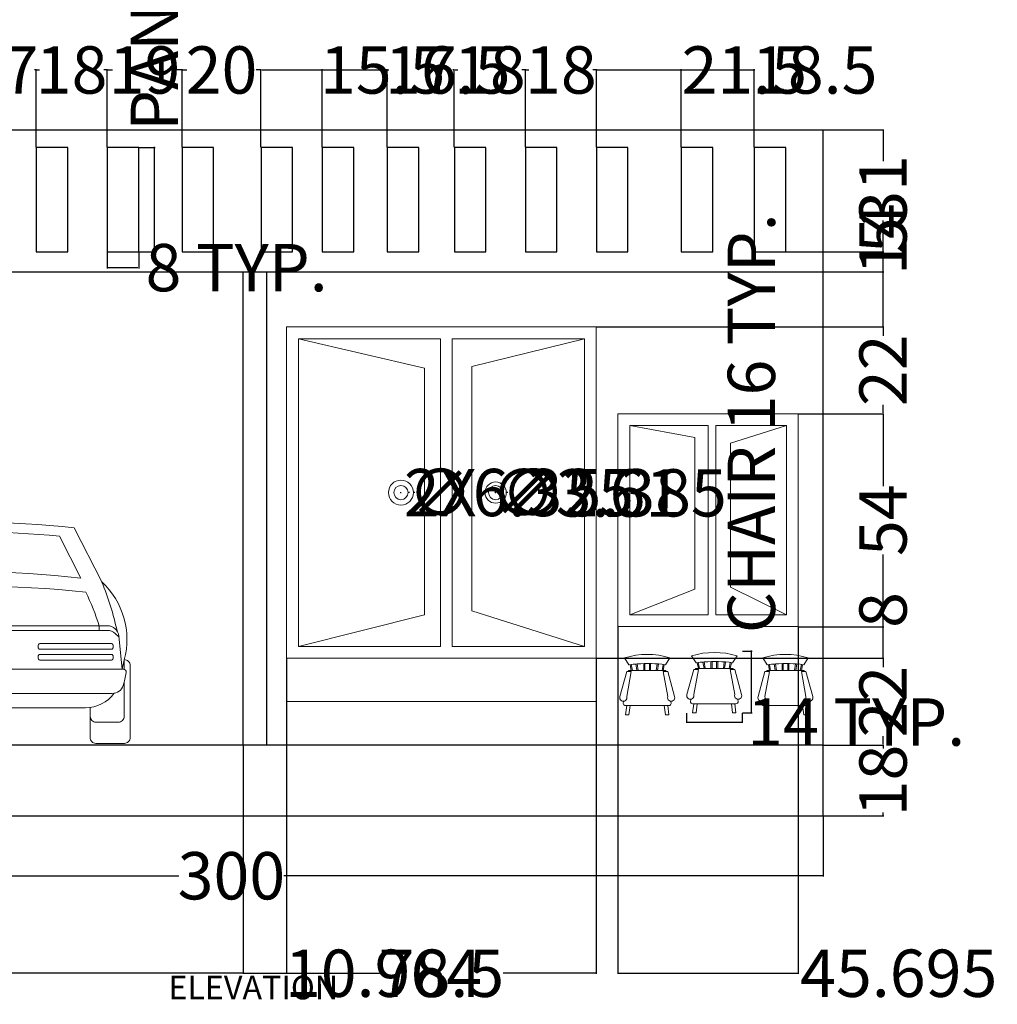
# Model space of a CAD drawing. Units: inches. Extents: x -101 to 786, y 26 to 880.
# Tile 7 of 9: x 538 to 786, y 45 to 295. Entities that reach past the tile are written whole.
import ezdxf

# ---------------------------------------------------------------- set-up
doc = ezdxf.new("R2010")
doc.units = ezdxf.units.IN
doc.header["$MEASUREMENT"] = 0
for name, color, linetype, lineweight in [('A-ANNO-DIMS', 2, 'Continuous', 18), ('A-ANNO-TEXT', 7, 'Continuous', 25), ('A-DOOR', 4, 'Continuous', 20), ('A-ELEV', 7, 'Continuous', 30), ('A-EQPM-VEHC', 9, 'Continuous', 13), ('A-FLOR-STRS', 7, 'Continuous', 20), ('A-FURN', 8, 'Continuous', 13), ('A-GLAZ', 4, 'Continuous', 18)]:
    doc.layers.add(name, color=color, linetype=linetype, lineweight=lineweight)
doc.styles.get("Standard").update_dxf_attribs({"font": 'arial.ttf'})
doc.dimstyles.get("Standard").update_dxf_attribs({"dimtxt": 12, "dimasz": 0.18, "dimexe": 0.18, "dimexo": 0.0625, "dimgap": 0.09, "dimtad": 0, "dimdec": 1, "dimzin": 0, "dimdsep": 46, "dimlunit": 3, "dimtxsty": 'Standard', "dimcen": 0.09, "dimadec": 0, "dimazin": 0, "dimtfac": 1, "dimtdec": 1, "dimtofl": 0, "dimtmove": 0, "dimatfit": 3, "dimfxl": 1, "dimtolj": 1, "dimtzin": 0, "dimarcsym": 0})

# ---------------------------------------------------------------- blocks, each defined once
blk = doc.blocks.new('*U16')
for p, q in [((-24.66, 54.68), (-31.66, 40.93)), ((31.66, 40.93), (24.66, 54.68)), ((-30.95, 37.96), (-30.95, 37.96)), ((-37.32, 21.22), (-36.82, 18.83)), ((36.82, 18.83), (37.31, 21.2)), ((-27.55, 9), (27.55, 9))]:
    blk.add_line(p, q)
for points in [[(-20.92, 52.5), (-26.31, 41.89), (-26.31, 41.89, -0.059427), (26.31, 41.89), (20.92, 52.5, 0.05217)], [(-34.12, 25.29), (-15.92, 25.29, -0.414214), (-15.55, 24.92), (-15.55, 24.24, -0.414214), (-15.92, 23.87), (-34.12, 23.87, -0.414214), (-34.49, 24.24), (-34.49, 24.92, -0.414214)], [(-2.82, 25.12), (2.9, 25.12, -0.414214), (3.64, 24.38), (3.64, 20.97, -0.414214), (2.9, 20.23), (-2.82, 20.23, -0.414214), (-3.56, 20.97), (-3.56, 24.38, -0.414214)], [(34.12, 25.29), (15.92, 25.29, 0.414214), (15.55, 24.92), (15.55, 24.24, 0.414214), (15.92, 23.87), (34.12, 23.87, 0.414214), (34.49, 24.24), (34.49, 24.92, 0.414214)], [(-34.12, 22.54), (-15.92, 22.54, -0.414214), (-15.55, 22.17), (-15.55, 21.49, -0.414214), (-15.92, 21.12), (-34.12, 21.12, -0.414214), (-34.49, 21.49), (-34.49, 22.17, -0.414214)], [(34.12, 22.54), (15.92, 22.54, 0.414214), (15.55, 22.17), (15.55, 21.49, 0.414214), (15.92, 21.12), (34.12, 21.12, 0.414214), (34.49, 21.49), (34.49, 22.17, 0.414214)], [(-7.5, 16.83, -0.414214), (-7, 17.33), (7, 17.33, -0.414214), (7.5, 16.83), (7.5, 13.67, 0.414214), (8.5, 12.67), (34.29, 12.67, 0.322734), (37.1, 14.69, 0.029256), (37.41, 15.83), (37.84, 17.94, 0.475639), (37.12, 18.83), (9, 18.83, -0.414214), (8.75, 19.08, 0.414214), (8.5, 19.33), (-8.5, 19.33, 0.414214), (-8.75, 19.08, -0.414214), (-9, 18.83), (-37.12, 18.83, 0.475639), (-37.84, 17.94), (-37.41, 15.83, 0.029158), (-37.1, 14.7, 0.322842), (-34.29, 12.67), (-8.5, 12.67, 0.414214), (-7.5, 13.67)]]:
    blk.add_lwpolyline(points, format="xyb", close=True)
for points in [[(30.95, 28.64), (30.95, 29.82, 0.037308), (27.62, 38.34, 0.052989), (-27.62, 38.34, 0.037308), (-30.95, 29.82), (-30.95, 28.64)], [(-36.82, 18.83), (-35.99, 27.2, -0.380946), (-33.05, 29.82), (33.04, 29.82, -0.380474), (35.98, 27.2), (36.82, 18.83)], [(-36.02, 26.89), (-35.02, 27.89, -0.184023), (-33.05, 28.64), (33.05, 28.64, -0.184023), (35.02, 27.89), (36.02, 26.89)], [(-28.73, 9.08), (-28.73, 1.48, -0.414214), (-30.21, 0), (-37.44, 0, -0.414214), (-38.92, 1.48), (-38.92, 19.74, -0.414214), (-37.44, 21.22), (-37.32, 21.22)], [(28.67, 9.07), (28.67, 1.48, 0.414214), (30.15, 0), (37.38, 0, 0.414214), (38.86, 1.48), (38.86, 19.74, 0.414214), (37.38, 21.22), (37.32, 21.22)], [(-37.32, 15.44), (-37.32, 6.85, 0.414214), (-35.84, 5.37), (-30.21, 5.37, 0.414214), (-28.73, 6.85), (-28.73, 9.08)], [(37.32, 15.44), (37.32, 6.85, -0.414214), (35.84, 5.37), (30.21, 5.37, -0.414214), (28.73, 6.85), (28.73, 9.08)]]:
    blk.add_lwpolyline(points, format="xyb")
for points in [[(-37.32, 21.22), (-37.32, 18.8)], [(37.32, 21.22), (37.32, 18.8)]]:
    blk.add_lwpolyline(points)
blk.add_circle((0, 26.18), 0.596)
for centre, radius, start, end in [((0, -181.13), 237.1, 84.03, 95.97), ((-18.4, 26.45), 19.63, 132.4835, 195.4658), ((30.86, 14.66), 67.81, 157.2124, 168.2366), ((18.26, 26.38), 19.77, 344.8595, 47.3598), ((-31.75, 14.41), 68.72, 11.827, 22.6625), ((-27.55, 17.88), 8.88, 215.5776, 270.0028), ((27.55, 17.88), 8.88, 270.0028, 324.3999)]:
    blk.add_arc(centre, radius, start, end)
blk = doc.blocks.new('Chair - Rocking')
for p, q in [((-8, -4.5), (-10, -1.5)), ((-4.5, -7), (-4.96674, -4.19951)), ((-4, -7), (-4.40532, -4.16272)), ((-1.5, -4.05012), (-1.5, -7)), ((-1, -7), (-1, -4.05012)), ((1, -7), (1, -4.04655)), ((1.5, -4.05012), (1.5, -7)), ((4, -7), (4.40187, -4.18694)), ((4.5, -7), (4.96761, -4.19437)), ((8, -4.5), (10, -1.5)), ((-9, -7.5), (-12, -18.49999)), ((-7, -7.5), (-9, -7.5)), ((-9, -18.49999), (-7, -7.5)), ((-8.23428, -6.99939), (-8.3093, -7.47958)), ((-8.23041, -7), (8.23915, -7)), ((-7.5, -4.5), (-7, -7)), ((-6.5, -7), (-7.02225, -4.43)), ((6.5, -7), (7, -4.4057)), ((7.5, -4.5), (7, -7)), ((7, -7.5), (9, -7.5)), ((9, -18.49999), (7, -7.5)), ((8.31071, -7.48854), (8.23449, -7.00073)), ((9, -7.5), (12, -18.49999)), ((-10.36644, -20.64523), (-10.5, -21.49999)), ((10.5, -21.49999), (10.3575, -20.58798)), ((-9, -22.49999), (-9.5, -26.49999)), ((0, -22.49999), (-9.5, -22.49999)), ((-8, -26.49999), (-7.5, -22.49999)), ((0, -22.49999), (9.5, -22.49999)), ((8, -26.49999), (7.5, -22.49999)), ((9, -22.49999), (9.5, -26.49999)), ((-9.5, -26.49999), (-8, -26.49999)), ((9.5, -26.49999), (8, -26.49999))]:
    blk.add_line(p, q)
for centre, radius, start, end in [((0, -34.08333), 34.08333, 72.93847, 107.0615), ((0, -68.25004), 64.25, 93.92211, 97.15267), ((0, -68.25004), 64.25, 82.84733, 93.92211), ((-10.5, -18.99999), 1.58114, 161.5651, 18.43495), ((-9.5, -21.49999), 1, 180, 270), ((10.5, -18.99999), 1.58114, 161.5651, 18.43495), ((9.5, -21.49999), 1, 270, 0)]:
    blk.add_arc(centre, radius, start, end)
blk = doc.blocks.new('PARAPET-PANEL-8')
blk.add_lwpolyline([(0, 0), (8, 0), (8, 26.5), (0, 26.5)], close=True)
blk = doc.blocks.new('*D27')
at = {"layer": 'A-ANNO-DIMS', "color": 0, "lineweight": -2, "transparency": 16777216}
for p, q in [((568.37, 262.42), (572.47, 262.42)), ((572.29, 262.42), (572.29, 262.6)), ((572.29, 236.1), (572.29, 262.24)), ((568.37, 235.92), (572.47, 235.92))]:
    blk.add_line(p, q, dxfattribs=at)
at = {"layer": 'A-ANNO-DIMS', "color": 0, "transparency": 16777216}
for points in [[(572.26, 262.24), (572.32, 262.24), (572.29, 262.42)], [(572.26, 236.1), (572.32, 236.1), (572.29, 235.92)]]:
    blk.add_solid(points, dxfattribs=at)
at = {"layer": 'Defpoints', "color": 0, "transparency": 16777216}
for p in [(568.31, 262.42), (572.29, 262.42), (568.31, 235.92)]:
    blk.add_point(p, dxfattribs=at)
at = {"layer": 'A-ANNO-DIMS', "color": 0, "transparency": 16777216, "insert": (572.29, 321.42), "char_height": 12, "attachment_point": 5, "rotation": 90}
blk.add_mtext('\\A1;PANEL 27 TYP.', dxfattribs=at)
blk = doc.blocks.new('*D28')
at = {"layer": 'A-ANNO-DIMS', "color": 0, "lineweight": -2, "transparency": 16777216}
for p, q in [((560.31, 235.86), (560.31, 231.77)), ((568.31, 235.86), (568.31, 231.77)), ((560.49, 231.95), (568.13, 231.95)), ((568.31, 231.95), (568.49, 231.95))]:
    blk.add_line(p, q, dxfattribs=at)
at = {"layer": 'A-ANNO-DIMS', "color": 0, "transparency": 16777216}
for points in [[(560.49, 231.98), (560.49, 231.92), (560.31, 231.95)], [(568.13, 231.98), (568.13, 231.92), (568.31, 231.95)]]:
    blk.add_solid(points, dxfattribs=at)
at = {"layer": 'Defpoints', "color": 0, "transparency": 16777216}
for p in [(560.31, 235.92), (568.31, 235.92), (568.31, 231.95)]:
    blk.add_point(p, dxfattribs=at)
at = {"layer": 'A-ANNO-DIMS', "color": 0, "transparency": 16777216, "insert": (593.13, 231.95), "char_height": 12, "attachment_point": 5}
blk.add_mtext('\\A1;8 TYP.', dxfattribs=at)
blk = doc.blocks.new('*D33')
at = {"layer": 'A-ANNO-DIMS', "color": 0, "lineweight": -2, "transparency": 16777216}
for p, q in [((723.59, 134.67), (723.59, 134.85)), ((721.31, 134.67), (723.77, 134.67)), ((723.59, 119.27), (723.59, 134.49)), ((721.31, 119.09), (723.77, 119.09))]:
    blk.add_line(p, q, dxfattribs=at)
at = {"layer": 'A-ANNO-DIMS', "color": 0, "transparency": 16777216}
for points in [[(723.56, 134.49), (723.62, 134.49), (723.59, 134.67)], [(723.56, 119.27), (723.62, 119.27), (723.59, 119.09)]]:
    blk.add_solid(points, dxfattribs=at)
at = {"layer": 'Defpoints', "color": 0, "transparency": 16777216}
for p in [(721.25, 134.67), (723.59, 134.67), (721.25, 119.09)]:
    blk.add_point(p, dxfattribs=at)
at = {"layer": 'A-ANNO-DIMS', "color": 0, "transparency": 16777216, "insert": (723.59, 192.49), "char_height": 12, "attachment_point": 5, "rotation": 90}
blk.add_mtext('\\A1;CHAIR 16 TYP.', dxfattribs=at)
blk = doc.blocks.new('*D34')
at = {"layer": 'A-ANNO-DIMS', "color": 0, "lineweight": -2, "transparency": 16777216}
for p, q in [((707.15, 119.02), (707.15, 116.57)), ((721.25, 119.02), (721.25, 116.57)), ((707.33, 116.75), (721.07, 116.75)), ((721.25, 116.75), (721.43, 116.75))]:
    blk.add_line(p, q, dxfattribs=at)
at = {"layer": 'A-ANNO-DIMS', "color": 0, "transparency": 16777216}
for points in [[(707.33, 116.78), (707.33, 116.72), (707.15, 116.75)], [(721.07, 116.78), (721.07, 116.72), (721.25, 116.75)]]:
    blk.add_solid(points, dxfattribs=at)
at = {"layer": 'Defpoints', "color": 0, "transparency": 16777216}
for p in [(707.15, 119.09), (721.25, 119.09), (721.25, 116.75)]:
    blk.add_point(p, dxfattribs=at)
at = {"layer": 'A-ANNO-DIMS', "color": 0, "transparency": 16777216, "insert": (750.16, 116.75), "char_height": 12, "attachment_point": 5}
blk.add_mtext('\\A1;14 TYP.', dxfattribs=at)
blk = doc.blocks.new('*D89')
at = {"layer": 'A-ANNO-DIMS', "color": 0, "lineweight": -2, "transparency": 16777216}
for p, q in [((441.81, 92.86), (441.81, 77.59)), ((741.81, 92.86), (741.81, 77.59)), ((441.99, 77.77), (578.49, 77.77)), ((741.63, 77.77), (605.13, 77.77))]:
    blk.add_line(p, q, dxfattribs=at)
at = {"layer": 'A-ANNO-DIMS', "color": 0, "transparency": 16777216}
for points in [[(441.99, 77.8), (441.99, 77.74), (441.81, 77.77)], [(741.63, 77.8), (741.63, 77.74), (741.81, 77.77)]]:
    blk.add_solid(points, dxfattribs=at)
at = {"layer": 'Defpoints', "color": 0, "transparency": 16777216}
for p in [(441.81, 92.92), (741.81, 92.92), (441.81, 77.77)]:
    blk.add_point(p, dxfattribs=at)
at = {"layer": 'A-ANNO-DIMS', "color": 0, "transparency": 16777216, "insert": (591.81, 77.77), "char_height": 12, "attachment_point": 5}
blk.add_mtext('\\A1;300', dxfattribs=at)
blk = doc.blocks.new('*D95')
at = {"layer": 'A-ANNO-DIMS', "color": 0, "lineweight": -2, "transparency": 16777216}
for p, q in [((525.31, 262.49), (525.31, 282.25)), ((542.31, 262.49), (542.31, 282.25)), ((525.49, 282.07), (525.69, 282.07)), ((542.13, 282.07), (541.93, 282.07))]:
    blk.add_line(p, q, dxfattribs=at)
at = {"layer": 'A-ANNO-DIMS', "color": 0, "transparency": 16777216}
for points in [[(525.49, 282.1), (525.49, 282.04), (525.31, 282.07)], [(542.13, 282.1), (542.13, 282.04), (542.31, 282.07)]]:
    blk.add_solid(points, dxfattribs=at)
at = {"layer": 'Defpoints', "color": 0, "transparency": 16777216}
for p in [(542.31, 282.07), (525.31, 262.42), (542.31, 262.42)]:
    blk.add_point(p, dxfattribs=at)
at = {"layer": 'A-ANNO-DIMS', "color": 0, "transparency": 16777216, "insert": (533.81, 282.07), "char_height": 12, "attachment_point": 5}
blk.add_mtext('\\A1;17', dxfattribs=at)
blk = doc.blocks.new('*D96')
at = {"layer": 'A-ANNO-DIMS', "color": 0, "lineweight": -2, "transparency": 16777216}
for p, q in [((542.31, 262.49), (542.31, 282.25)), ((560.31, 262.49), (560.31, 282.25)), ((542.49, 282.07), (543.18, 282.07)), ((560.13, 282.07), (559.44, 282.07))]:
    blk.add_line(p, q, dxfattribs=at)
at = {"layer": 'A-ANNO-DIMS', "color": 0, "transparency": 16777216}
for points in [[(542.49, 282.1), (542.49, 282.04), (542.31, 282.07)], [(560.13, 282.1), (560.13, 282.04), (560.31, 282.07)]]:
    blk.add_solid(points, dxfattribs=at)
at = {"layer": 'Defpoints', "color": 0, "transparency": 16777216}
for p in [(560.31, 282.07), (542.31, 262.42), (560.31, 262.42)]:
    blk.add_point(p, dxfattribs=at)
at = {"layer": 'A-ANNO-DIMS', "color": 0, "transparency": 16777216, "insert": (551.31, 282.07), "char_height": 12, "attachment_point": 5}
blk.add_mtext('\\A1;18', dxfattribs=at)
blk = doc.blocks.new('*D97')
at = {"layer": 'A-ANNO-DIMS', "color": 0, "lineweight": -2, "transparency": 16777216}
for p, q in [((560.31, 262.49), (560.31, 282.25)), ((579.31, 262.49), (579.31, 282.25)), ((560.49, 282.07), (561.68, 282.07)), ((579.13, 282.07), (577.94, 282.07))]:
    blk.add_line(p, q, dxfattribs=at)
at = {"layer": 'A-ANNO-DIMS', "color": 0, "transparency": 16777216}
for points in [[(560.49, 282.1), (560.49, 282.04), (560.31, 282.07)], [(579.13, 282.1), (579.13, 282.04), (579.31, 282.07)]]:
    blk.add_solid(points, dxfattribs=at)
at = {"layer": 'Defpoints', "color": 0, "transparency": 16777216}
for p in [(579.31, 282.07), (560.31, 262.42), (579.31, 262.42)]:
    blk.add_point(p, dxfattribs=at)
at = {"layer": 'A-ANNO-DIMS', "color": 0, "transparency": 16777216, "insert": (569.81, 282.07), "char_height": 12, "attachment_point": 5}
blk.add_mtext('\\A1;19', dxfattribs=at)
blk = doc.blocks.new('*D98')
at = {"layer": 'A-ANNO-DIMS', "color": 0, "lineweight": -2, "transparency": 16777216}
for p, q in [((579.31, 262.49), (579.31, 282.25)), ((599.31, 262.49), (599.31, 282.25)), ((579.49, 282.07), (580.55, 282.07)), ((599.13, 282.07), (598.08, 282.07))]:
    blk.add_line(p, q, dxfattribs=at)
at = {"layer": 'A-ANNO-DIMS', "color": 0, "transparency": 16777216}
for points in [[(579.49, 282.1), (579.49, 282.04), (579.31, 282.07)], [(599.13, 282.1), (599.13, 282.04), (599.31, 282.07)]]:
    blk.add_solid(points, dxfattribs=at)
at = {"layer": 'Defpoints', "color": 0, "transparency": 16777216}
for p in [(599.31, 282.07), (579.31, 262.42), (599.31, 262.42)]:
    blk.add_point(p, dxfattribs=at)
at = {"layer": 'A-ANNO-DIMS', "color": 0, "transparency": 16777216, "insert": (589.31, 282.07), "char_height": 12, "attachment_point": 5}
blk.add_mtext('\\A1;20', dxfattribs=at)
blk = doc.blocks.new('*D99')
at = {"layer": 'A-ANNO-DIMS', "color": 0, "lineweight": -2, "transparency": 16777216}
for p, q in [((599.31, 262.49), (599.31, 282.25)), ((614.81, 262.49), (614.81, 282.25)), ((599.49, 282.07), (614.63, 282.07)), ((614.81, 282.07), (614.99, 282.07))]:
    blk.add_line(p, q, dxfattribs=at)
at = {"layer": 'A-ANNO-DIMS', "color": 0, "transparency": 16777216}
for points in [[(599.49, 282.1), (599.49, 282.04), (599.31, 282.07)], [(614.63, 282.1), (614.63, 282.04), (614.81, 282.07)]]:
    blk.add_solid(points, dxfattribs=at)
at = {"layer": 'Defpoints', "color": 0, "transparency": 16777216}
for p in [(614.81, 282.07), (599.31, 262.42), (614.81, 262.42)]:
    blk.add_point(p, dxfattribs=at)
at = {"layer": 'A-ANNO-DIMS', "color": 0, "transparency": 16777216, "insert": (630.15, 282.07), "char_height": 12, "attachment_point": 5}
blk.add_mtext('\\A1;15.5', dxfattribs=at)
blk = doc.blocks.new('*D100')
at = {"layer": 'A-ANNO-DIMS', "color": 0, "lineweight": -2, "transparency": 16777216}
for p, q in [((614.81, 262.49), (614.81, 282.25)), ((631.31, 262.49), (631.31, 282.25)), ((614.99, 282.07), (631.13, 282.07)), ((631.31, 282.07), (631.49, 282.07))]:
    blk.add_line(p, q, dxfattribs=at)
at = {"layer": 'A-ANNO-DIMS', "color": 0, "transparency": 16777216}
for points in [[(614.99, 282.1), (614.99, 282.04), (614.81, 282.07)], [(631.13, 282.1), (631.13, 282.04), (631.31, 282.07)]]:
    blk.add_solid(points, dxfattribs=at)
at = {"layer": 'Defpoints', "color": 0, "transparency": 16777216}
for p in [(631.31, 282.07), (614.81, 262.42), (631.31, 262.42)]:
    blk.add_point(p, dxfattribs=at)
at = {"layer": 'A-ANNO-DIMS', "color": 0, "transparency": 16777216, "insert": (646.65, 282.07), "char_height": 12, "attachment_point": 5}
blk.add_mtext('\\A1;16.5', dxfattribs=at)
blk = doc.blocks.new('*D101')
at = {"layer": 'A-ANNO-DIMS', "color": 0, "lineweight": -2, "transparency": 16777216}
for p, q in [((631.31, 262.49), (631.31, 282.25)), ((648.31, 262.49), (648.31, 282.25)), ((631.49, 282.07), (631.69, 282.07)), ((648.13, 282.07), (647.93, 282.07))]:
    blk.add_line(p, q, dxfattribs=at)
at = {"layer": 'A-ANNO-DIMS', "color": 0, "transparency": 16777216}
for points in [[(631.49, 282.1), (631.49, 282.04), (631.31, 282.07)], [(648.13, 282.1), (648.13, 282.04), (648.31, 282.07)]]:
    blk.add_solid(points, dxfattribs=at)
at = {"layer": 'Defpoints', "color": 0, "transparency": 16777216}
for p in [(648.31, 282.07), (631.31, 262.42), (648.31, 262.42)]:
    blk.add_point(p, dxfattribs=at)
at = {"layer": 'A-ANNO-DIMS', "color": 0, "transparency": 16777216, "insert": (639.81, 282.07), "char_height": 12, "attachment_point": 5}
blk.add_mtext('\\A1;17', dxfattribs=at)
blk = doc.blocks.new('*D102')
at = {"layer": 'A-ANNO-DIMS', "color": 0, "lineweight": -2, "transparency": 16777216}
for p, q in [((648.31, 262.49), (648.31, 282.25)), ((666.31, 262.49), (666.31, 282.25)), ((648.49, 282.07), (649.18, 282.07)), ((666.13, 282.07), (665.44, 282.07))]:
    blk.add_line(p, q, dxfattribs=at)
at = {"layer": 'A-ANNO-DIMS', "color": 0, "transparency": 16777216}
for points in [[(648.49, 282.1), (648.49, 282.04), (648.31, 282.07)], [(666.13, 282.1), (666.13, 282.04), (666.31, 282.07)]]:
    blk.add_solid(points, dxfattribs=at)
at = {"layer": 'Defpoints', "color": 0, "transparency": 16777216}
for p in [(666.31, 282.07), (648.31, 262.42), (666.31, 262.42)]:
    blk.add_point(p, dxfattribs=at)
at = {"layer": 'A-ANNO-DIMS', "color": 0, "transparency": 16777216, "insert": (657.31, 282.07), "char_height": 12, "attachment_point": 5}
blk.add_mtext('\\A1;18', dxfattribs=at)
blk = doc.blocks.new('*D103')
at = {"layer": 'A-ANNO-DIMS', "color": 0, "lineweight": -2, "transparency": 16777216}
for p, q in [((666.31, 262.49), (666.31, 282.25)), ((684.31, 262.49), (684.31, 282.25)), ((666.49, 282.07), (667.18, 282.07)), ((684.13, 282.07), (683.44, 282.07))]:
    blk.add_line(p, q, dxfattribs=at)
at = {"layer": 'A-ANNO-DIMS', "color": 0, "transparency": 16777216}
for points in [[(666.49, 282.1), (666.49, 282.04), (666.31, 282.07)], [(684.13, 282.1), (684.13, 282.04), (684.31, 282.07)]]:
    blk.add_solid(points, dxfattribs=at)
at = {"layer": 'Defpoints', "color": 0, "transparency": 16777216}
for p in [(684.31, 282.07), (666.31, 262.42), (684.31, 262.42)]:
    blk.add_point(p, dxfattribs=at)
at = {"layer": 'A-ANNO-DIMS', "color": 0, "transparency": 16777216, "insert": (675.31, 282.07), "char_height": 12, "attachment_point": 5}
blk.add_mtext('\\A1;18', dxfattribs=at)
blk = doc.blocks.new('*D104')
at = {"layer": 'A-ANNO-DIMS', "color": 0, "lineweight": -2, "transparency": 16777216}
for p, q in [((684.31, 262.49), (684.31, 282.25)), ((705.81, 262.49), (705.81, 282.25)), ((684.49, 282.07), (705.63, 282.07)), ((705.81, 282.07), (705.99, 282.07))]:
    blk.add_line(p, q, dxfattribs=at)
at = {"layer": 'A-ANNO-DIMS', "color": 0, "transparency": 16777216}
for points in [[(684.49, 282.1), (684.49, 282.04), (684.31, 282.07)], [(705.63, 282.1), (705.63, 282.04), (705.81, 282.07)]]:
    blk.add_solid(points, dxfattribs=at)
at = {"layer": 'Defpoints', "color": 0, "transparency": 16777216}
for p in [(705.81, 282.07), (684.31, 262.42), (705.81, 262.42)]:
    blk.add_point(p, dxfattribs=at)
at = {"layer": 'A-ANNO-DIMS', "color": 0, "transparency": 16777216, "insert": (721.81, 282.07), "char_height": 12, "attachment_point": 5}
blk.add_mtext('\\A1;21.5', dxfattribs=at)
blk = doc.blocks.new('*D105')
at = {"layer": 'A-ANNO-DIMS', "color": 0, "lineweight": -2, "transparency": 16777216}
for p, q in [((705.81, 262.49), (705.81, 282.25)), ((724.31, 262.49), (724.31, 282.25)), ((705.99, 282.07), (724.13, 282.07)), ((724.31, 282.07), (724.49, 282.07))]:
    blk.add_line(p, q, dxfattribs=at)
at = {"layer": 'A-ANNO-DIMS', "color": 0, "transparency": 16777216}
for points in [[(705.99, 282.1), (705.99, 282.04), (705.81, 282.07)], [(724.13, 282.1), (724.13, 282.04), (724.31, 282.07)]]:
    blk.add_solid(points, dxfattribs=at)
at = {"layer": 'Defpoints', "color": 0, "transparency": 16777216}
for p in [(724.31, 282.07), (705.81, 262.42), (724.31, 262.42)]:
    blk.add_point(p, dxfattribs=at)
at = {"layer": 'A-ANNO-DIMS', "color": 0, "transparency": 16777216, "insert": (739.65, 282.07), "char_height": 12, "attachment_point": 5}
blk.add_mtext('\\A1;18.5', dxfattribs=at)
blk = doc.blocks.new('*D107')
at = {"layer": 'A-ANNO-DIMS', "color": 0, "lineweight": -2, "transparency": 16777216}
for p, q in [((741.87, 110.92), (757.14, 110.92)), ((756.96, 110.74), (756.96, 110.06)), ((741.87, 92.92), (757.14, 92.92)), ((756.96, 93.1), (756.96, 93.79))]:
    blk.add_line(p, q, dxfattribs=at)
at = {"layer": 'A-ANNO-DIMS', "color": 0, "transparency": 16777216}
for points in [[(756.93, 110.74), (756.99, 110.74), (756.96, 110.92)], [(756.93, 93.1), (756.99, 93.1), (756.96, 92.92)]]:
    blk.add_solid(points, dxfattribs=at)
at = {"layer": 'Defpoints', "color": 0, "transparency": 16777216}
for p in [(741.81, 110.92), (756.96, 110.92), (741.81, 92.92)]:
    blk.add_point(p, dxfattribs=at)
at = {"layer": 'A-ANNO-DIMS', "color": 0, "transparency": 16777216, "insert": (756.96, 101.92), "char_height": 12, "attachment_point": 5, "rotation": 90}
blk.add_mtext('\\A1;18', dxfattribs=at)
blk = doc.blocks.new('*D108')
at = {"layer": 'A-ANNO-DIMS', "color": 0, "lineweight": -2, "transparency": 16777216}
for p, q in [((684.34, 132.92), (757.14, 132.92)), ((756.96, 132.74), (756.96, 130.65)), ((756.96, 111.1), (756.96, 113.2)), ((741.87, 110.92), (757.14, 110.92))]:
    blk.add_line(p, q, dxfattribs=at)
at = {"layer": 'A-ANNO-DIMS', "color": 0, "transparency": 16777216}
for points in [[(756.93, 132.74), (756.99, 132.74), (756.96, 132.92)], [(756.93, 111.1), (756.99, 111.1), (756.96, 110.92)]]:
    blk.add_solid(points, dxfattribs=at)
at = {"layer": 'Defpoints', "color": 0, "transparency": 16777216}
for p in [(684.28, 132.92), (756.96, 132.92), (741.81, 110.92)]:
    blk.add_point(p, dxfattribs=at)
at = {"layer": 'A-ANNO-DIMS', "color": 0, "transparency": 16777216, "insert": (756.96, 121.92), "char_height": 12, "attachment_point": 5, "rotation": 90}
blk.add_mtext('\\A1;22', dxfattribs=at)
blk = doc.blocks.new('*D109')
at = {"layer": 'A-ANNO-DIMS', "color": 0, "lineweight": -2, "transparency": 16777216}
for p, q in [((735.53, 140.92), (757.14, 140.92)), ((756.96, 140.92), (756.96, 141.1)), ((756.96, 133.1), (756.96, 140.74)), ((684.34, 132.92), (757.14, 132.92))]:
    blk.add_line(p, q, dxfattribs=at)
at = {"layer": 'A-ANNO-DIMS', "color": 0, "transparency": 16777216}
for points in [[(756.93, 140.74), (756.99, 140.74), (756.96, 140.92)], [(756.93, 133.1), (756.99, 133.1), (756.96, 132.92)]]:
    blk.add_solid(points, dxfattribs=at)
at = {"layer": 'Defpoints', "color": 0, "transparency": 16777216}
for p in [(735.47, 140.92), (756.96, 140.92), (684.28, 132.92)]:
    blk.add_point(p, dxfattribs=at)
at = {"layer": 'A-ANNO-DIMS', "color": 0, "transparency": 16777216, "insert": (756.96, 145.15), "char_height": 12, "attachment_point": 5, "rotation": 90}
blk.add_mtext('\\A1;8', dxfattribs=at)
blk = doc.blocks.new('*D110')
at = {"layer": 'A-ANNO-DIMS', "color": 0, "lineweight": -2, "transparency": 16777216}
for p, q in [((735.53, 194.92), (757.14, 194.92)), ((756.96, 194.74), (756.96, 176.58)), ((756.96, 141.1), (756.96, 159.26)), ((735.53, 140.92), (757.14, 140.92))]:
    blk.add_line(p, q, dxfattribs=at)
at = {"layer": 'A-ANNO-DIMS', "color": 0, "transparency": 16777216}
for points in [[(756.93, 194.74), (756.99, 194.74), (756.96, 194.92)], [(756.93, 141.1), (756.99, 141.1), (756.96, 140.92)]]:
    blk.add_solid(points, dxfattribs=at)
at = {"layer": 'Defpoints', "color": 0, "transparency": 16777216}
for p in [(735.47, 194.92), (756.96, 194.92), (735.47, 140.92)]:
    blk.add_point(p, dxfattribs=at)
at = {"layer": 'A-ANNO-DIMS', "color": 0, "transparency": 16777216, "insert": (756.96, 167.92), "char_height": 12, "attachment_point": 5, "rotation": 90}
blk.add_mtext('\\A1;54', dxfattribs=at)
blk = doc.blocks.new('*D111')
at = {"layer": 'A-ANNO-DIMS', "color": 0, "lineweight": -2, "transparency": 16777216}
for p, q in [((684.34, 216.92), (757.14, 216.92)), ((756.96, 216.74), (756.96, 214.65)), ((735.53, 194.92), (757.14, 194.92)), ((756.96, 195.1), (756.96, 197.2))]:
    blk.add_line(p, q, dxfattribs=at)
at = {"layer": 'A-ANNO-DIMS', "color": 0, "transparency": 16777216}
for points in [[(756.93, 216.74), (756.99, 216.74), (756.96, 216.92)], [(756.93, 195.1), (756.99, 195.1), (756.96, 194.92)]]:
    blk.add_solid(points, dxfattribs=at)
at = {"layer": 'Defpoints', "color": 0, "transparency": 16777216}
for p in [(684.28, 216.92), (756.96, 216.92), (735.47, 194.92)]:
    blk.add_point(p, dxfattribs=at)
at = {"layer": 'A-ANNO-DIMS', "color": 0, "transparency": 16777216, "insert": (756.96, 205.92), "char_height": 12, "attachment_point": 5, "rotation": 90}
blk.add_mtext('\\A1;22', dxfattribs=at)
blk = doc.blocks.new('*D112')
at = {"layer": 'A-ANNO-DIMS', "color": 0, "lineweight": -2, "transparency": 16777216}
for p, q in [((741.87, 230.92), (757.14, 230.92)), ((756.96, 230.92), (756.96, 231.1)), ((756.96, 217.1), (756.96, 230.74)), ((684.34, 216.92), (757.14, 216.92))]:
    blk.add_line(p, q, dxfattribs=at)
at = {"layer": 'A-ANNO-DIMS', "color": 0, "transparency": 16777216}
for points in [[(756.93, 230.74), (756.99, 230.74), (756.96, 230.92)], [(756.93, 217.1), (756.99, 217.1), (756.96, 216.92)]]:
    blk.add_solid(points, dxfattribs=at)
at = {"layer": 'Defpoints', "color": 0, "transparency": 16777216}
for p in [(741.81, 230.92), (756.96, 230.92), (684.28, 216.92)]:
    blk.add_point(p, dxfattribs=at)
at = {"layer": 'A-ANNO-DIMS', "color": 0, "transparency": 16777216, "insert": (756.96, 239.2), "char_height": 12, "attachment_point": 5, "rotation": 90}
blk.add_mtext('\\A1;14', dxfattribs=at)
blk = doc.blocks.new('*D113')
at = {"layer": 'A-ANNO-DIMS', "color": 0, "lineweight": -2, "transparency": 16777216}
for p, q in [((732.37, 235.92), (757.14, 235.92)), ((756.96, 235.92), (756.96, 236.1)), ((756.96, 231.1), (756.96, 235.74)), ((741.87, 230.92), (757.14, 230.92))]:
    blk.add_line(p, q, dxfattribs=at)
at = {"layer": 'A-ANNO-DIMS', "color": 0, "transparency": 16777216}
for points in [[(756.93, 235.74), (756.99, 235.74), (756.96, 235.92)], [(756.93, 231.1), (756.99, 231.1), (756.96, 230.92)]]:
    blk.add_solid(points, dxfattribs=at)
at = {"layer": 'Defpoints', "color": 0, "transparency": 16777216}
for p in [(732.31, 235.92), (756.96, 235.92), (741.81, 230.92)]:
    blk.add_point(p, dxfattribs=at)
at = {"layer": 'A-ANNO-DIMS', "color": 0, "transparency": 16777216, "insert": (756.96, 240.17), "char_height": 12, "attachment_point": 5, "rotation": 90}
blk.add_mtext('\\A1;5', dxfattribs=at)
blk = doc.blocks.new('*D114')
at = {"layer": 'A-ANNO-DIMS', "color": 0, "lineweight": -2, "transparency": 16777216}
for p, q in [((741.87, 266.92), (757.14, 266.92)), ((756.96, 266.74), (756.96, 258.95)), ((756.96, 236.1), (756.96, 243.9)), ((732.37, 235.92), (757.14, 235.92))]:
    blk.add_line(p, q, dxfattribs=at)
at = {"layer": 'A-ANNO-DIMS', "color": 0, "transparency": 16777216}
for points in [[(756.93, 266.74), (756.99, 266.74), (756.96, 266.92)], [(756.93, 236.1), (756.99, 236.1), (756.96, 235.92)]]:
    blk.add_solid(points, dxfattribs=at)
at = {"layer": 'Defpoints', "color": 0, "transparency": 16777216}
for p in [(741.81, 266.92), (756.96, 266.92), (732.31, 235.92)]:
    blk.add_point(p, dxfattribs=at)
at = {"layer": 'A-ANNO-DIMS', "color": 0, "transparency": 16777216, "insert": (756.96, 251.42), "char_height": 12, "attachment_point": 5, "rotation": 90}
blk.add_mtext('\\A1;31', dxfattribs=at)
blk = doc.blocks.new('*D115')
at = {"layer": 'A-ANNO-DIMS', "color": 0, "lineweight": -2, "transparency": 16777216}
for p, q in [((450.81, 110.86), (450.81, 52.87)), ((594.81, 110.86), (594.81, 52.87)), ((450.99, 53.05), (510.05, 53.05)), ((594.63, 53.05), (535.57, 53.05))]:
    blk.add_line(p, q, dxfattribs=at)
at = {"layer": 'A-ANNO-DIMS', "color": 0, "transparency": 16777216}
for points in [[(450.99, 53.08), (450.99, 53.02), (450.81, 53.05)], [(594.63, 53.08), (594.63, 53.02), (594.81, 53.05)]]:
    blk.add_solid(points, dxfattribs=at)
at = {"layer": 'Defpoints', "color": 0, "transparency": 16777216}
for p in [(450.81, 110.92), (594.81, 110.92), (594.81, 53.05)]:
    blk.add_point(p, dxfattribs=at)
at = {"layer": 'A-ANNO-DIMS', "color": 0, "transparency": 16777216, "insert": (522.81, 53.05), "char_height": 12, "attachment_point": 5}
blk.add_mtext('\\A1;144', dxfattribs=at)
blk = doc.blocks.new('*D116')
at = {"layer": 'A-ANNO-DIMS', "color": 0, "lineweight": -2, "transparency": 16777216}
for p, q in [((605.78, 132.86), (605.78, 52.87)), ((594.81, 110.86), (594.81, 52.87)), ((594.99, 53.05), (605.6, 53.05)), ((605.78, 53.05), (605.96, 53.05))]:
    blk.add_line(p, q, dxfattribs=at)
at = {"layer": 'A-ANNO-DIMS', "color": 0, "transparency": 16777216}
for points in [[(594.99, 53.08), (594.99, 53.02), (594.81, 53.05)], [(605.6, 53.08), (605.6, 53.02), (605.78, 53.05)]]:
    blk.add_solid(points, dxfattribs=at)
at = {"layer": 'Defpoints', "color": 0, "transparency": 16777216}
for p in [(605.78, 132.92), (594.81, 110.92), (605.78, 53.05)]:
    blk.add_point(p, dxfattribs=at)
at = {"layer": 'A-ANNO-DIMS', "color": 0, "transparency": 16777216, "insert": (630.36, 53.05), "char_height": 12, "attachment_point": 5}
blk.add_mtext('\\A1;10.964', dxfattribs=at)
blk = doc.blocks.new('*D117')
at = {"layer": 'A-ANNO-DIMS', "color": 0, "lineweight": -2, "transparency": 16777216}
for p, q in [((605.78, 132.86), (605.78, 52.87)), ((684.28, 132.86), (684.28, 52.87)), ((605.96, 53.05), (629.35, 53.05)), ((684.1, 53.05), (660.7, 53.05))]:
    blk.add_line(p, q, dxfattribs=at)
at = {"layer": 'A-ANNO-DIMS', "color": 0, "transparency": 16777216}
for points in [[(605.96, 53.08), (605.96, 53.02), (605.78, 53.05)], [(684.1, 53.08), (684.1, 53.02), (684.28, 53.05)]]:
    blk.add_solid(points, dxfattribs=at)
at = {"layer": 'Defpoints', "color": 0, "transparency": 16777216}
for p in [(605.78, 132.92), (684.28, 132.92), (684.28, 53.05)]:
    blk.add_point(p, dxfattribs=at)
at = {"layer": 'A-ANNO-DIMS', "color": 0, "transparency": 16777216, "insert": (645.03, 53.05), "char_height": 12, "attachment_point": 5}
blk.add_mtext('\\A1;78.5', dxfattribs=at)
blk = doc.blocks.new('*D118')
at = {"layer": 'A-ANNO-DIMS', "color": 0, "lineweight": -2, "transparency": 16777216}
for p, q in [((689.78, 140.86), (689.78, 52.87)), ((735.47, 140.86), (735.47, 52.87)), ((689.96, 53.05), (735.29, 53.05)), ((735.47, 53.05), (735.65, 53.05))]:
    blk.add_line(p, q, dxfattribs=at)
at = {"layer": 'A-ANNO-DIMS', "color": 0, "transparency": 16777216}
for points in [[(689.96, 53.08), (689.96, 53.02), (689.78, 53.05)], [(735.29, 53.08), (735.29, 53.02), (735.47, 53.05)]]:
    blk.add_solid(points, dxfattribs=at)
at = {"layer": 'Defpoints', "color": 0, "transparency": 16777216}
for p in [(689.78, 140.92), (735.47, 140.92), (735.47, 53.05)]:
    blk.add_point(p, dxfattribs=at)
at = {"layer": 'A-ANNO-DIMS', "color": 0, "transparency": 16777216, "insert": (760.94, 53.05), "char_height": 12, "attachment_point": 5}
blk.add_mtext('\\A1;45.695', dxfattribs=at)
blk = doc.blocks.new('*D133')
at = {"layer": 'A-ANNO-DIMS', "color": 0, "lineweight": -2, "transparency": 16777216}
for p, q in [((634.69, 174.92), (634.87, 174.92)), ((634.78, 174.83), (634.78, 175.01)), ((638.3, 174.92), (638.12, 174.92))]:
    blk.add_line(p, q, dxfattribs=at)
at = {"layer": 'A-ANNO-DIMS', "color": 0, "transparency": 16777216}
blk.add_solid([(638.12, 174.95), (638.12, 174.89), (637.94, 174.92)], dxfattribs=at)
at = {"layer": 'Defpoints', "color": 0, "transparency": 16777216}
for p in [(631.61, 174.92), (637.94, 174.92)]:
    blk.add_point(p, dxfattribs=at)
at = {"layer": 'A-ANNO-DIMS', "color": 0, "transparency": 16777216, "insert": (665.21, 174.93), "char_height": 12, "attachment_point": 5, "rotation": 0.0038}
blk.add_mtext('\\A1;∅6.325', dxfattribs=at)
blk = doc.blocks.new('*D134')
at = {"layer": 'A-ANNO-DIMS', "color": 0, "lineweight": -2, "transparency": 16777216}
for p, q in [((658.69, 174.92), (658.87, 174.92)), ((658.78, 174.83), (658.78, 175.01)), ((661.83, 174.92), (661.65, 174.92))]:
    blk.add_line(p, q, dxfattribs=at)
at = {"layer": 'A-ANNO-DIMS', "color": 0, "transparency": 16777216}
blk.add_solid([(661.65, 174.95), (661.65, 174.89), (661.47, 174.92)], dxfattribs=at)
at = {"layer": 'Defpoints', "color": 0, "transparency": 16777216}
for p in [(656.08, 174.93), (661.47, 174.92)]:
    blk.add_point(p, dxfattribs=at)
at = {"layer": 'A-ANNO-DIMS', "color": 0, "transparency": 16777216, "insert": (688.74, 174.88), "char_height": 12, "attachment_point": 5, "rotation": 359.9203}
blk.add_mtext('\\A1;∅5.385', dxfattribs=at)
blk = doc.blocks.new('*D135')
at = {"layer": 'A-ANNO-DIMS', "color": 0, "lineweight": -2, "transparency": 16777216}
for p, q in [((634.69, 174.92), (634.87, 174.92)), ((634.78, 174.83), (634.78, 175.01)), ((636.94, 174.92), (636.76, 174.92))]:
    blk.add_line(p, q, dxfattribs=at)
at = {"layer": 'A-ANNO-DIMS', "color": 0, "transparency": 16777216}
blk.add_solid([(636.76, 174.95), (636.76, 174.89), (636.58, 174.92)], dxfattribs=at)
at = {"layer": 'Defpoints', "color": 0, "transparency": 16777216}
for p in [(632.97, 174.93), (636.58, 174.92)]:
    blk.add_point(p, dxfattribs=at)
at = {"layer": 'A-ANNO-DIMS', "color": 0, "transparency": 16777216, "insert": (670.66, 174.85), "char_height": 12, "attachment_point": 5, "rotation": 359.8796}
blk.add_mtext('\\A1;2X ∅3.61', dxfattribs=at)

msp = doc.modelspace()

# ---------------------------------------------------------------- linework, layer by layer
at = {"layer": 'A-DOOR'}
for p, q in [((608.7756, 213.9238), (644.7756, 213.9238)), ((608.7756, 135.9238), (608.7756, 213.9238)), ((608.7756, 213.9238), (640.7756, 206.4238)), ((644.7756, 135.9238), (644.7756, 213.9238)), ((647.7756, 135.9238), (647.7756, 213.9238)), ((647.7756, 213.9238), (681.2756, 213.9238)), ((681.2756, 213.9238), (652.7756, 206.9238)), ((681.2756, 213.9238), (681.2756, 135.9238)), ((640.7756, 206.4238), (640.7756, 143.9238)), ((652.7756, 206.9238), (652.7756, 144.9238)), ((652.7756, 144.9238), (681.2756, 135.9238)), ((640.7756, 143.9238), (608.7756, 135.9238)), ((644.7756, 135.9238), (608.7756, 135.9238)), ((681.2756, 135.9238), (647.7756, 135.9238))]:
    msp.add_line(p, q, dxfattribs=at)
msp.add_lwpolyline([(605.7756, 216.9238), (684.2756, 216.9238), (684.2756, 132.9238), (605.7756, 132.9238)], close=True, dxfattribs=at)
for centre, radius in [((634.7756, 174.9238), 3.1623), ((658.7756, 174.9238), 2.6926), ((658.7756, 174.9238), 2.6926), ((658.7756, 174.9238), 2.6926), ((658.7756, 174.9238), 2.6926), ((634.7756, 174.9238), 1.8028), ((658.7756, 174.9238), 1.8028)]:
    msp.add_circle(centre, radius, dxfattribs=at)
at = {"layer": 'A-ELEV'}
for p, q in [((441.8117, 266.9238), (741.8117, 266.9238)), ((741.8117, 92.9238), (741.8117, 266.9238)), ((441.8117, 230.9238), (741.8117, 230.9238)), ((594.8117, 110.9238), (594.8117, 230.9238)), ((600.8117, 110.9238), (600.8117, 230.9238)), ((441.8117, 110.9238), (741.8117, 110.9238)), ((441.8117, 92.9238), (741.8117, 92.9238))]:
    msp.add_line(p, q, dxfattribs=at)
at = {"layer": 'A-FLOR-STRS'}
for p, q in [((605.7756, 121.9238), (605.7756, 132.9238)), ((684.2756, 121.9238), (684.2756, 132.9238)), ((605.7756, 121.9238), (684.2756, 121.9238)), ((605.7756, 121.9238), (605.7756, 110.9238)), ((684.2756, 121.9238), (684.2756, 110.9238))]:
    msp.add_line(p, q, dxfattribs=at)
at = {"layer": 'A-GLAZ'}
for p, q in [((692.7756, 191.9238), (709.2756, 188.9238)), ((712.6232, 191.9238), (712.6232, 143.9238)), ((714.6232, 191.9238), (714.6232, 143.9238)), ((732.4709, 191.9238), (718.2756, 187.4238)), ((709.2756, 188.9238), (709.2756, 150.4238)), ((718.2756, 187.4238), (718.2756, 150.9238)), ((709.2756, 150.4238), (692.7756, 143.9238)), ((718.2756, 150.9238), (732.4709, 143.9238))]:
    msp.add_line(p, q, dxfattribs=at)
msp.add_lwpolyline([(689.7756, 140.9238), (689.7756, 194.9238), (735.4709, 194.9238), (735.4709, 140.9238)], close=True, dxfattribs=at)
for points in [[(712.6232, 143.9238), (692.7756, 143.9238), (692.7756, 191.9238), (712.6232, 191.9238)], [(714.6232, 191.9238), (732.4709, 191.9238), (732.4709, 143.9238), (714.6232, 143.9238)]]:
    msp.add_lwpolyline(points, dxfattribs=at)

# ---------------------------------------------------------------- block references
at = {"layer": 'A-ELEV'}
for p in [(542.312, 235.924), (560.312, 235.924), (579.312, 235.924), (599.312, 235.924), (614.812, 235.924), (631.312, 235.924), (648.312, 235.924), (666.312, 235.924), (684.312, 235.924), (705.812, 235.924), (724.312, 235.924)]:
    msp.add_blockref('PARAPET-PANEL-8', p, dxfattribs=at)
at = {"layer": 'A-EQPM-VEHC'}
msp.add_blockref('*U16', (527.3117, 111.3367), dxfattribs=at)
at = {"layer": 'A-FURN', "xscale": 0.5772621950364011, "yscale": 0.5772621950364011, "zscale": 0.5772621950364011}
for p in [(697.1983, 133.883), (714.1983, 134.383), (732.2345, 133.883)]:
    msp.add_blockref('Chair - Rocking', p, dxfattribs=at)

# ---------------------------------------------------------------- texts
at = {"layer": 'A-ANNO-TEXT'}
msp.add_text('ELEVATION', height=6, dxfattribs=at).set_placement((575.8117, 46.4238))

# ---------------------------------------------------------------- dimensions: what is measured, and where the dimension line sits
at = {"layer": 'A-ANNO-DIMS'}
for base, p1, p2, text, picture, middle in [((572.2867420758, 262.4237895654), (568.3117420758, 235.9237895654), (568.3117420758, 262.4237895654), 'PANEL <> TYP.', '*D27', (572.2867420758, 321.4168454999)), ((723.589, 134.6716), (721.251, 119.0855), (721.251, 134.6716), 'CHAIR <> TYP.', '*D33', (723.589, 192.4859))]:
    dim = msp.add_linear_dim(base=base, p1=p1, p2=p2, angle=90, text=text, dimstyle='Standard', override={"dimdec": 0, "dimlfac": 1, "dimrnd": 0, "dimzin": 0, "dimdsep": 46, "dimlunit": 2}, dxfattribs=at)
    dim.commit()
    dim.dimension.update_dxf_attribs({"geometry": picture, "text_midpoint": middle})
for base, p1, p2, override, picture, middle in [((542.3117, 282.0738), (525.3117, 262.4238), (542.3117, 262.4238), {"dimdec": 0, "dimlfac": 1, "dimrnd": 0, "dimzin": 0, "dimdsep": 46, "dimlunit": 2}, '*D95', (533.8117, 282.0738)), ((560.3117, 282.0738), (542.3117, 262.4238), (560.3117, 262.4238), {"dimdec": 0, "dimlfac": 1, "dimrnd": 0, "dimzin": 0, "dimdsep": 46, "dimlunit": 2}, '*D96', (551.3117, 282.0738)), ((579.3117, 282.0738), (560.3117, 262.4238), (579.3117, 262.4238), {"dimdec": 0, "dimlfac": 1, "dimrnd": 0, "dimzin": 0, "dimdsep": 46, "dimlunit": 2}, '*D97', (569.8117, 282.0738)), ((599.3117, 282.0738), (579.3117, 262.4238), (599.3117, 262.4238), {"dimdec": 0, "dimlfac": 1, "dimrnd": 0, "dimzin": 0, "dimdsep": 46, "dimlunit": 2}, '*D98', (589.3117, 282.0738)), ((614.8117, 282.0738), (599.3117, 262.4238), (614.8117, 262.4238), {"dimdec": 1, "dimlfac": 1, "dimrnd": 0, "dimzin": 0, "dimdsep": 46, "dimlunit": 2}, '*D99', (630.1472, 282.0738)), ((631.3117, 282.0738), (614.8117, 262.4238), (631.3117, 262.4238), {"dimdec": 1, "dimlfac": 1, "dimrnd": 0, "dimzin": 0, "dimdsep": 46, "dimlunit": 2}, '*D100', (646.6472, 282.0738)), ((648.3117, 282.0738), (631.3117, 262.4238), (648.3117, 262.4238), {"dimdec": 0, "dimlfac": 1, "dimrnd": 0, "dimzin": 0, "dimdsep": 46, "dimlunit": 2}, '*D101', (639.8117, 282.0738)), ((666.3117, 282.0738), (648.3117, 262.4238), (666.3117, 262.4238), {"dimdec": 0, "dimlfac": 1, "dimrnd": 0, "dimzin": 0, "dimdsep": 46, "dimlunit": 2}, '*D102', (657.3117, 282.0738)), ((684.3117, 282.0738), (666.3117, 262.4238), (684.3117, 262.4238), {"dimdec": 0, "dimlfac": 1, "dimrnd": 0, "dimzin": 0, "dimdsep": 46, "dimlunit": 2}, '*D103', (675.3117, 282.0738)), ((705.8117, 282.0738), (684.3117, 262.4238), (705.8117, 262.4238), {"dimdec": 1, "dimlfac": 1, "dimrnd": 0, "dimzin": 0, "dimdsep": 46, "dimlunit": 2}, '*D104', (721.8143, 282.0738)), ((724.3117, 282.0738), (705.8117, 262.4238), (724.3117, 262.4238), {"dimdec": 1, "dimlfac": 1, "dimrnd": 0, "dimzin": 0, "dimdsep": 46, "dimlunit": 2}, '*D105', (739.6472, 282.0738)), ((735.4709, 53.0498), (689.7756, 140.9238), (735.4709, 140.9238), {"dimdec": 3, "dimlfac": 1, "dimrnd": 0, "dimzin": 0, "dimdsep": 46, "dimlunit": 2}, '*D118', (760.936, 53.0498)), ((605.7756, 53.0498), (594.8117, 110.9238), (605.7756, 132.9238), {"dimdec": 3, "dimlfac": 1, "dimrnd": 0, "dimzin": 0, "dimdsep": 46, "dimlunit": 2}, '*D116', (630.3648, 53.0498)), ((684.2756, 53.0498), (605.7756, 132.9238), (684.2756, 132.9238), {"dimdec": 1, "dimlfac": 1, "dimrnd": 0, "dimzin": 0, "dimdsep": 46, "dimlunit": 2}, '*D117', (645.0256, 53.0498)), ((594.8117, 53.0498), (450.8117, 110.9238), (594.8117, 110.9238), {"dimdec": 0, "dimlfac": 1, "dimrnd": 0, "dimzin": 0, "dimdsep": 46, "dimlunit": 2}, '*D115', (522.8117, 53.0498))]:
    dim = msp.add_linear_dim(base=base, p1=p1, p2=p2, dimstyle='Standard', override=override, dxfattribs=at)
    dim.commit()
    dim.dimension.update_dxf_attribs({"geometry": picture, "text_midpoint": middle})
for base, p1, p2, angle, picture, middle in [((756.9617, 266.9238), (732.3117, 235.9238), (741.8117, 266.9238), 90, '*D114', (756.9617, 251.4238)), ((756.9617, 230.9238), (684.2756, 216.9238), (741.8117, 230.9238), 90, '*D112', (756.9617, 239.1992)), ((756.9617, 235.9238), (741.8117, 230.9238), (732.3117, 235.9238), 90, '*D113', (756.9617, 240.172)), ((756.9617, 216.9238), (735.4709, 194.9238), (684.2756, 216.9238), 90, '*D111', (756.9617, 205.9238)), ((756.9617, 194.9238), (735.4709, 140.9238), (735.4709, 194.9238), 90, '*D110', (756.9617, 167.9238)), ((756.9617, 140.9238), (684.2756, 132.9238), (735.4709, 140.9238), 90, '*D109', (756.9617, 145.1474)), ((756.9617, 132.9238), (741.8117, 110.9238), (684.2756, 132.9238), 90, '*D108', (756.9617, 121.9238)), ((756.9617, 110.9238), (741.8117, 92.9238), (741.8117, 110.9238), 90, '*D107', (756.9617, 101.9238)), ((441.8117, 77.7738), (741.8117, 92.9238), (441.8117, 92.9238), 180, '*D89', (591.8117, 77.7738))]:
    dim = msp.add_linear_dim(base=base, p1=p1, p2=p2, angle=angle, dimstyle='Standard', override={"dimdec": 0, "dimlfac": 1, "dimrnd": 0, "dimzin": 0, "dimdsep": 46, "dimlunit": 2}, dxfattribs=at)
    dim.commit()
    dim.dimension.update_dxf_attribs({"geometry": picture, "text_midpoint": middle})
for base, p1, p2, picture, middle in [((568.3117, 231.9488), (560.3117, 235.9238), (568.3117, 235.9238), '*D28', (593.1343, 231.9488)), ((721.251, 116.7476), (707.1456, 119.0855), (721.251, 119.0855), '*D34', (750.1622, 116.7476))]:
    dim = msp.add_linear_dim(base=base, p1=p1, p2=p2, text='<> TYP.', dimstyle='Standard', override={"dimdec": 0, "dimlfac": 1, "dimrnd": 0, "dimzin": 0, "dimdsep": 46, "dimlunit": 2}, dxfattribs=at)
    dim.commit()
    dim.dimension.update_dxf_attribs({"geometry": picture, "text_midpoint": middle})
dim = msp.add_diameter_dim_2p(p1=(632.9728, 174.9276), p2=(636.5784, 174.92), text='2X <>', dimstyle='Standard', override={"dimdec": 2, "dimlfac": 1, "dimrnd": 0, "dimzin": 0, "dimdsep": 46, "dimlunit": 2}, dxfattribs=at)
dim.commit()
dim.dimension.update_dxf_attribs({"geometry": '*D135', "text_midpoint": (670.6586, 174.8484), "dimtype": 163})
dim = msp.add_diameter_dim_2p(p1=(631.6133, 174.9236), p2=(637.9379, 174.924), dimstyle='Standard', override={"dimdec": 3, "dimlfac": 1, "dimrnd": 0, "dimzin": 0, "dimdsep": 46, "dimlunit": 2}, dxfattribs=at)
dim.commit()
dim.dimension.update_dxf_attribs({"geometry": '*D133', "text_midpoint": (665.2078, 174.9258), "dimtype": 163})
dim = msp.add_diameter_dim_2p(p1=(656.083, 174.9275), p2=(661.4682, 174.92), dimstyle='Standard', override={"dimdec": 3, "dimlfac": 1, "dimrnd": 0, "dimzin": 0, "dimdsep": 46, "dimlunit": 2}, dxfattribs=at)
dim.commit()
dim.dimension.update_dxf_attribs({"geometry": '*D134', "text_midpoint": (688.7381, 174.8821)})

doc.saveas('drawing.dxf')
